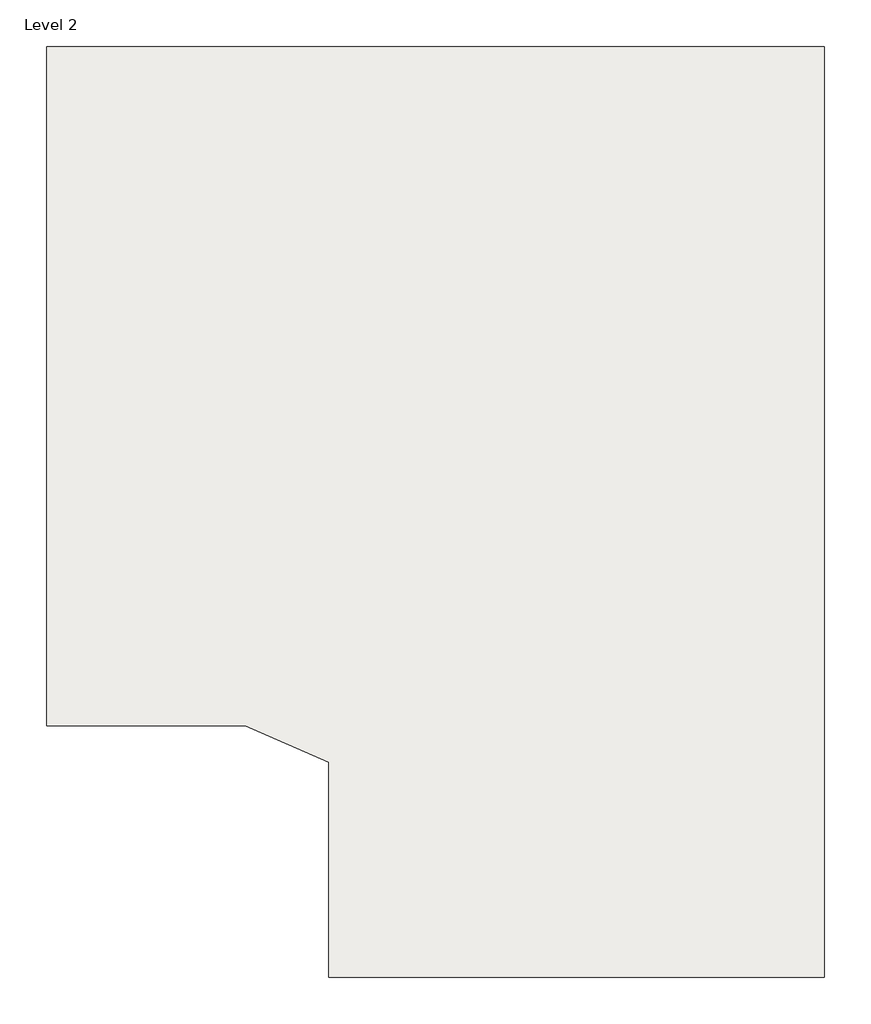
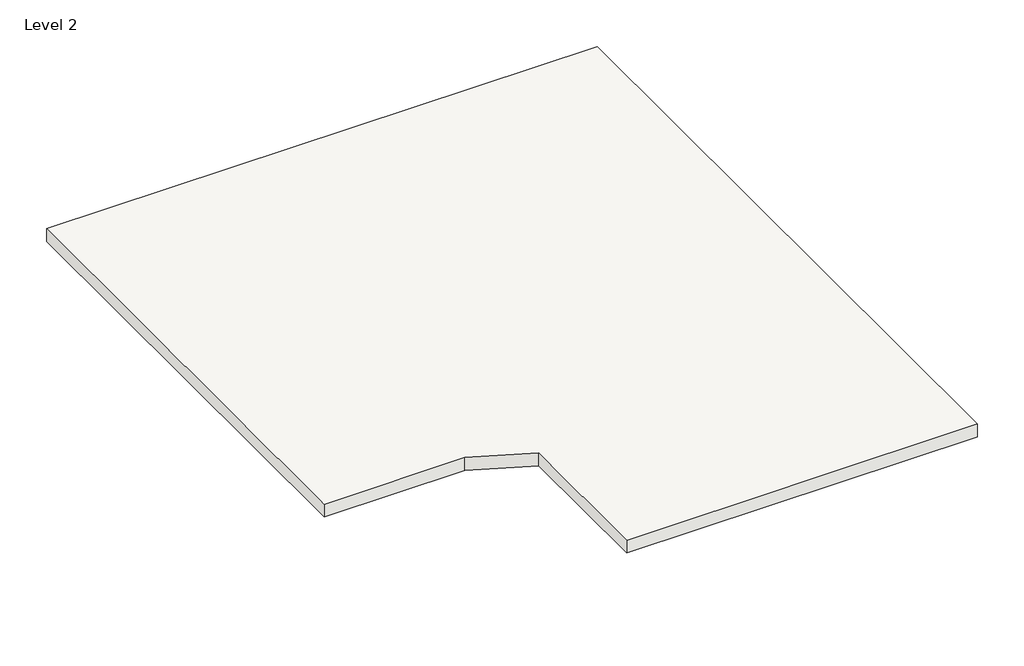
# One storey: 1 roof.
"""IFC4 building model written with IfcOpenShell, lengths in millimetres."""

from ifc_helpers import new_model, si_unit, frame, origin, place, context, project, spatial, polyline, outline, extrude, element, save

model = new_model("IFC4")

# Units and contexts
model_context = context("Model", 3, world=origin())
ifc_project = project(units=[si_unit("LENGTHUNIT", "METRE", prefix="MILLI")], contexts=[model_context])

# Site, building, storey
site = spatial("IfcSite", under=ifc_project)
building = spatial("IfcBuilding", under=site)
storey = spatial("IfcBuildingStorey", under=building, Name="Level 2", Elevation=3048.0)

# Roof
placement = place(None, origin())
element("IfcRoof", 1, ObjectType="Generic - 12\"", at=placement, inside=storey, context=model_context, shape_type="SweptSolid", body=[
    extrude(outline(polyline([(-14976.2744419, 13927.0452409), (-2581.0744419, 13927.0452409), (-2581.0744419, -906.5547591), (-10480.4744419, -906.5547591), (-10480.4744419, 2522.4452409), (-11807.1406807, 3106.6452409), (-14976.2744419, 3106.6452409), (-14976.2744419, 13927.0452409)])), frame((0.0, 0.0, 3048.0), z_axis=(0.0, 0.0, 1.0), x_axis=(1.0, 0.0, 0.0)), (0.0, 0.0, 1.0), 304.8),
])

save(model, "model.ifc")

# Revit data of these elements
# Type "Generic - 12\""
#   Assembly Code = "B1020"
#   Layers, outside or top first: 1' - 0" "Brick, Soldier Course" (function 1)
# Element 1 (IfcRoof, "Generic - 12\"")
#   built-in parameter 1001705 = 11 (stored number, unit not read)
#   built-in parameter 1001710 = 33615
#   Phase Created = New Construction
#   Materials on its faces: "Brick, Soldier Course"
# Materials
#   "Brick, Soldier Course": class "Masonry", colour RGB 170 98 104, transparency 0, Description = "Common brick soldier coursed", Cost = 0
